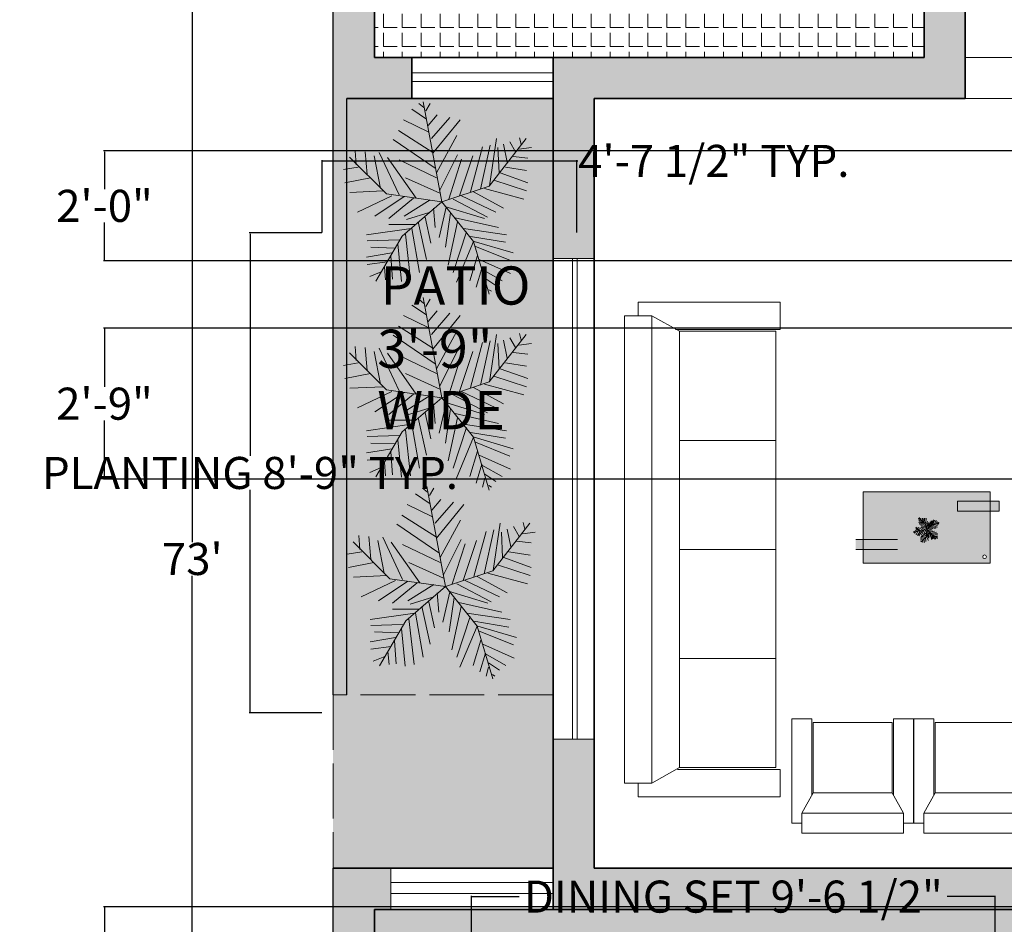
# Model space of a CAD drawing. Units: inches. Extents: x 1884 to 2398, y 474 to 1488.
# Tile 32 of 39: x 1884 to 2099, y 889 to 1087. Entities that reach past the tile are written whole.
import ezdxf

# ---------------------------------------------------------------- set-up
doc = ezdxf.new("R2010")
doc.units = ezdxf.units.IN
doc.header["$MEASUREMENT"] = 0
doc.linetypes.add('ACAD_ISO02W100', pattern=[15, 12, -3])
doc.layers.get('0').update_dxf_attribs({"color": 250})
for name, color, linetype, lineweight in [('A-ANNO-DIMS', 2, 'Continuous', 18), ('A-AREA-IDEN', 7, 'Continuous', 18), ('A-FLOR-OVHD', 8, 'ACAD_ISO02W100', 18), ('A-FLOR-PATT', 254, 'Continuous', 13), ('A-FURN-PATT', 253, 'Continuous', 13), ('A-WALL-PATT', 250, 'Continuous', 13), ('C-PROP', 7, 'Continuous', 30), ('furniture', 8, 'Continuous', 18), ('L-PLNT', 73, 'Continuous', 18), ('walls', 7, 'Continuous', 35), ('windows', 4, 'Continuous', 18)]:
    doc.layers.add(name, color=color, linetype=linetype, lineweight=lineweight)
doc.layers.add('L-PVMT-PATT', color=9, linetype='Continuous', lineweight=13, true_color=0xc7c8ca)
doc.styles.get("Standard").update_dxf_attribs({"font": 'arial.ttf'})
doc.dimstyles.get("Standard").update_dxf_attribs({"dimtxt": 7, "dimasz": 0.18, "dimexe": 0.18, "dimexo": 0.0625, "dimgap": 0.09, "dimtad": 0, "dimtih": 1, "dimtoh": 1, "dimzin": 0, "dimdsep": 46, "dimlunit": 3, "dimtxsty": 'Standard', "dimcen": 0.09, "dimadec": 0, "dimazin": 0, "dimtfac": 1, "dimtofl": 0, "dimtmove": 0, "dimatfit": 3, "dimfxl": 1, "dimtolj": 1, "dimtzin": 0, "dimarcsym": 0})

# ---------------------------------------------------------------- blocks, each defined once
blk = doc.blocks.new('*D2')
at = {"layer": 'A-ANNO-DIMS', "color": 0, "lineweight": -2, "transparency": 16777216}
for p, q in [((1920.51, 1406.88), (1921.96, 1406.88)), ((1921.78, 1406.7), (1921.78, 972.55)), ((1921.78, 531.06), (1921.78, 965.22)), ((1920.51, 530.88), (1921.96, 530.88))]:
    blk.add_line(p, q, dxfattribs=at)
at = {"layer": 'A-ANNO-DIMS', "color": 0, "lineweight": 100, "transparency": 16777216}
for points in [[(1921.75, 1406.7), (1921.81, 1406.7), (1921.78, 1406.88)], [(1921.75, 531.06), (1921.81, 531.06), (1921.78, 530.88)]]:
    blk.add_solid(points, dxfattribs=at)
at = {"layer": 'Defpoints', "color": 0, "lineweight": 100, "transparency": 16777216}
for p in [(1920.45, 1406.88), (1920.45, 530.88), (1921.78, 530.88)]:
    blk.add_point(p, dxfattribs=at)
at = {"layer": 'A-ANNO-DIMS', "color": 0, "transparency": 16777216, "insert": (1921.78, 968.88), "char_height": 7, "attachment_point": 5}
blk.add_mtext("\\A1;73'", dxfattribs=at)
blk = doc.blocks.new('tpoy')
at = {"layer": 'furniture'}
h = blk.add_hatch(color=256, dxfattribs=at)
h.dxf.hatch_style = 1
h.paths.add_polyline_path([(278.09, -251.06), (275.9, -251.06), (275.9, -258.19), (278.09, -258.19)])
h.paths.add_polyline_path([(278.09, -249.1), (275.9, -249.1), (275.9, -251.06), (278.09, -251.06)])
h.paths.add_polyline_path([(286.44, -271.28), (284.25, -271.28), (284.25, -278.76), (286.44, -278.76)])
h.paths.add_polyline_path([(286.44, -278.76), (284.25, -278.76), (284.25, -280.38), (286.44, -280.38)])
for p, q in [((275.9, -249.1), (278.09, -249.1)), ((275.9, -258.19), (275.9, -249.1)), ((278.09, -249.1), (278.09, -258.19)), ((273.86, -251.06), (273.86, -278.76)), ((289.38, -251.06), (273.86, -251.06)), ((289.38, -278.76), (289.38, -251.06)), ((278.09, -258.19), (275.9, -258.19)), ((284.25, -280.38), (284.25, -271.28)), ((286.44, -271.28), (286.44, -280.38)), ((273.86, -278.76), (289.38, -278.76))]:
    blk.add_line(p, q, dxfattribs=at)
blk.add_circle((288.03, -252.28), 0.401, dxfattribs=at)
blk = doc.blocks.new('*U20')
for p, q in [((-7.288, 39.707), (-21.778, 46.673)), ((-8.737, 47.138), (-17.069, 52.711)), ((-10.186, 53.64), (-13.084, 55.962)), ((0, 0), (-10.5, 57)), ((-9.099, 51.782), (-6.563, 55.962)), ((-7.65, 43.423), (-2.578, 49.46)), ((-5.839, 35.992), (4.667, 48.067)), ((-5.114, 27.632), (10.463, 46.673)), ((-47.498, 19.737), (-55.83, 18.344)), ((-40.615, 13.7), (-55.105, 10.913)), ((-31.5, 4.5), (-52.5, 25.5)), ((-33.37, 6.269), (-52.207, 5.34)), ((-48.585, 21.131), (-49.309, 29.026)), ((-28.299, 3.483), (-47.86, -5.805)), ((-43.513, 28.561), (-42.427, 15.558)), ((-38.442, 26.239), (-34.819, 7.663)), ((-21.416, 3.018), (-38.079, -8.128)), ((-35.544, 28.097), (-24.314, 3.947)), ((0, 0), (-31.5, 4.5)), ((-14.533, 2.09), (-30.834, 25.31)), ((-15.982, 2.09), (-30.11, -9.521)), ((-3.665, 19.273), (-27.574, 35.527)), ((-5.114, 28.097), (-24.676, 40.636)), ((-24.314, 23.917), (-2.941, 13.7)), ((0, 0), (-22.5, -19.5)), ((-6.563, 1.161), (-21.416, -8.128)), ((-20.691, 13.7), (-1.129, 4.876)), ((-2.941, 16.486), (8.652, 37.85)), ((-1.129, 6.734), (9.014, 26.704)), ((0, 0), (27, 9)), ((0, 0), (18, -22.5)), ((3.942, 1.625), (11.187, 24.381)), ((6.478, 1.625), (26.04, -8.592)), ((10.101, 3.483), (17.708, 26.239)), ((11.187, 3.483), (30.749, -5.805)), ((16.259, 5.805), (23.142, 31.348)), ((18.07, 5.805), (35.096, -3.483)), ((22.055, 7.198), (27.489, 32.277)), ((24.229, 7.663), (46.688, 1.625)), ((27, 9), (48, 36)), ((27.127, 9.056), (31.112, 35.992)), ((29.662, 12.307), (48.137, 6.269)), ((31.836, 30.883), (32.561, 16.486)), ((33.285, 16.486), (48.862, 10.913)), ((35.096, 32.741), (37.27, 22.524)), ((36.183, 19.737), (48.137, 17.88)), ((38.719, 34.134), (41.979, 28.561)), ((40.53, 25.775), (48.862, 24.846)), ((43.791, 29.954), (51.036, 30.883)), ((44.153, 36.456), (45.239, 32.741)), ((-17.431, -15.094), (-42.789, -18.809)), ((-28.299, -29.026), (-42.789, -31.348)), ((-24.314, -21.596), (-42.427, -22.06)), ((-30.834, -34.135), (-42.427, -35.528)), ((-34.457, -39.708), (-40.978, -42.494)), ((-26.849, -26.24), (-40.253, -25.775)), ((-22.5, -19.5), (-37.5, -45)), ((-32.646, -36.921), (-31.921, -44.352)), ((-15.257, -12.772), (-30.11, -12.772)), ((-29.023, -30.884), (-27.936, -43.887)), ((-25.038, -23.918), (-22.865, -45.281)), ((-20.691, -18.345), (-17.793, -44.352)), ((-6.563, -5.805), (-19.967, -9.985)), ((-17.069, -15.094), (-12.721, -40.172)), ((-13.446, -11.378), (-8.737, -32.741)), ((-9.461, -8.592), (-6.201, -23.453)), ((-4.752, -3.483), (-3.665, -14.629)), ((2.493, -3.019), (-1.491, -20.202)), ((1.769, -2.555), (24.229, -9.521)), ((5.029, -6.27), (2.131, -25.775)), ((9.014, -11.378), (3.58, -35.992)), ((14.085, -16.951), (6.478, -40.172)), ((7.565, -9.056), (32.198, -14.629)), ((18.07, -22.524), (8.289, -45.745)), ((12.274, -15.094), (36.907, -18.809)), ((20.244, -30.419), (15.897, -44.816)), ((16.259, -19.738), (36.183, -22.989)), ((18, -22.5), (27, -52.5)), ((18.433, -22.524), (40.53, -29.026)), ((19.157, -25.311), (38.719, -33.206)), ((22.78, -37.85), (19.519, -48.532)), ((21.331, -32.741), (39.081, -40.636)), ((22.78, -38.314), (34.372, -44.816)), ((24.591, -45.745), (23.142, -50.854)), ((24.591, -43.423), (30.749, -47.603)), ((26.764, -49.925), (28.213, -50.854))]:
    blk.add_line(p, q)
blk = doc.blocks.new('Trees - Imperial')
for p, q in [((0, 0), (-10.5, 57)), ((-8.737, 47.138), (-17.069, 52.711)), ((-10.186, 53.64), (-13.084, 55.962)), ((-9.099, 51.782), (-6.563, 55.962)), ((-7.288, 39.707), (-21.778, 46.673)), ((-7.65, 43.423), (-2.578, 49.46)), ((-5.839, 35.992), (4.667, 48.067)), ((-5.114, 27.632), (10.463, 46.673)), ((-5.114, 28.097), (-24.676, 40.636)), ((-3.665, 19.273), (-27.574, 35.527)), ((-2.941, 16.486), (8.652, 37.85)), ((27, 9), (48, 36)), ((27.127, 9.056), (31.112, 35.992)), ((38.719, 34.134), (41.979, 28.561)), ((44.153, 36.456), (45.239, 32.741)), ((-48.585, 21.131), (-49.309, 29.026)), ((-43.513, 28.561), (-42.427, 15.558)), ((-35.544, 28.097), (-24.314, 3.947)), ((16.259, 5.805), (23.142, 31.348)), ((22.055, 7.198), (27.489, 32.277)), ((31.836, 30.883), (32.561, 16.486)), ((35.096, 32.741), (37.27, 22.524)), ((43.791, 29.954), (51.036, 30.883)), ((-31.5, 4.5), (-52.5, 25.5)), ((-38.442, 26.239), (-34.819, 7.663)), ((-14.533, 2.09), (-30.834, 25.31)), ((-24.314, 23.917), (-2.941, 13.7)), ((-1.129, 6.734), (9.014, 26.704)), ((3.942, 1.625), (11.187, 24.381)), ((10.101, 3.483), (17.708, 26.239)), ((40.53, 25.775), (48.862, 24.846)), ((-47.498, 19.737), (-55.83, 18.344)), ((36.183, 19.737), (48.137, 17.88)), ((-40.615, 13.7), (-55.105, 10.913)), ((-20.691, 13.7), (-1.129, 4.876)), ((29.662, 12.307), (48.137, 6.269)), ((33.285, 16.486), (48.862, 10.913)), ((-33.37, 6.269), (-52.207, 5.34)), ((0, 0), (27, 9)), ((18.07, 5.805), (35.096, -3.483)), ((24.229, 7.663), (46.688, 1.625)), ((-28.299, 3.483), (-47.86, -5.805)), ((-21.416, 3.018), (-38.079, -8.128)), ((0, 0), (-31.5, 4.5)), ((-15.982, 2.09), (-30.11, -9.521)), ((0, 0), (-22.5, -19.5)), ((-6.563, 1.161), (-21.416, -8.128)), ((0, 0), (18, -22.5)), ((6.478, 1.625), (26.04, -8.592)), ((11.187, 3.483), (30.749, -5.805)), ((-4.752, -3.483), (-3.665, -14.629)), ((2.493, -3.019), (-1.491, -20.202)), ((1.769, -2.555), (24.229, -9.521)), ((-6.563, -5.805), (-19.967, -9.985)), ((-9.461, -8.592), (-6.201, -23.453)), ((5.029, -6.27), (2.131, -25.775)), ((7.565, -9.056), (32.198, -14.629)), ((-17.431, -15.094), (-42.789, -18.809)), ((-15.257, -12.772), (-30.11, -12.772)), ((-17.069, -15.094), (-12.721, -40.172)), ((-13.446, -11.378), (-8.737, -32.741)), ((9.014, -11.378), (3.58, -35.992)), ((12.274, -15.094), (36.907, -18.809)), ((-24.314, -21.596), (-42.427, -22.06)), ((-22.5, -19.5), (-37.5, -45)), ((-20.691, -18.345), (-17.793, -44.352)), ((14.085, -16.951), (6.478, -40.172)), ((16.259, -19.738), (36.183, -22.989)), ((-26.849, -26.24), (-40.253, -25.775)), ((-25.038, -23.918), (-22.865, -45.281)), ((18.07, -22.524), (8.289, -45.745)), ((18, -22.5), (27, -52.5)), ((18.433, -22.524), (40.53, -29.026)), ((19.157, -25.311), (38.719, -33.206)), ((-28.299, -29.026), (-42.789, -31.348)), ((-29.023, -30.884), (-27.936, -43.887)), ((20.244, -30.419), (15.897, -44.816)), ((21.331, -32.741), (39.081, -40.636)), ((-30.834, -34.135), (-42.427, -35.528)), ((-32.646, -36.921), (-31.921, -44.352)), ((22.78, -37.85), (19.519, -48.532)), ((22.78, -38.314), (34.372, -44.816)), ((-34.457, -39.708), (-40.978, -42.494)), ((24.591, -43.423), (30.749, -47.603)), ((24.591, -45.745), (23.142, -50.854)), ((26.764, -49.925), (28.213, -50.854))]:
    blk.add_line(p, q)
blk = doc.blocks.new('FABRIC SOFA 4S')
at = {"layer": 'furniture'}
for p, q in [((3, 54), (34, 54)), ((3, 51), (3, 54)), ((34, 48), (34, 54)), ((0, -51), (0, 51)), ((6, 51), (0, 51)), ((6, -51), (6, 51)), ((12, 47.63), (6, 51)), ((11.14, 48), (34, 48)), ((33, 23.81), (12, 23.81)), ((33, 0), (12, 0)), ((33, -23.81), (12, -23.81)), ((6, -51), (12, -47.63)), ((11.54, -48), (34, -48)), ((34, -48), (34, -54)), ((6, -51), (0, -51)), ((3, -54), (3, -51)), ((3, -54), (34, -54))]:
    blk.add_line(p, q, dxfattribs=at)
blk.add_lwpolyline([(12, -47.63), (12, 47.63), (33, 47.63), (33, -47.63)], close=True, dxfattribs=at)
blk = doc.blocks.new('FABRIC SOFA 1S')
at = {"layer": 'furniture'}
for p, q in [((3, 18.12), (34, 18.12)), ((3, 15.12), (3, 18.12)), ((34, 12.12), (34, 18.12)), ((0, -15.12), (0, 15.12)), ((6, 15.12), (0, 15.12)), ((6, -15.12), (6, 15.12)), ((12, 11.75), (6, 15.12)), ((11.33, 12.12), (34, 12.12)), ((6, -15.12), (12, -11.75)), ((11.33, -12.12), (34, -12.12)), ((34, -12.12), (34, -18.12)), ((6, -15.12), (0, -15.12)), ((3, -18.12), (3, -15.12)), ((3, -18.12), (34, -18.12))]:
    blk.add_line(p, q, dxfattribs=at)
blk.add_lwpolyline([(12, -11.75), (12, 11.75), (33, 11.75), (33, -11.75)], close=True, dxfattribs=at)
blk = doc.blocks.new('*D35')
at = {"layer": 'A-ANNO-DIMS', "color": 0, "lineweight": -2, "transparency": 16777216}
for p, q in [((1982.72, 878.09), (1982.72, 895.35)), ((1982.9, 895.17), (1993.17, 895.17)), ((2096.86, 895.17), (2086.6, 895.17)), ((2097.04, 878.09), (2097.04, 895.35))]:
    blk.add_line(p, q, dxfattribs=at)
at = {"layer": 'A-ANNO-DIMS', "color": 0, "lineweight": 100, "transparency": 16777216}
for points in [[(1982.9, 895.2), (1982.9, 895.14), (1982.72, 895.17)], [(2096.86, 895.2), (2096.86, 895.14), (2097.04, 895.17)]]:
    blk.add_solid(points, dxfattribs=at)
at = {"layer": 'Defpoints', "color": 0, "lineweight": 100, "transparency": 16777216}
for p in [(2097.04, 895.17), (1982.72, 878.02), (2097.04, 878.02)]:
    blk.add_point(p, dxfattribs=at)
at = {"layer": 'A-ANNO-DIMS', "color": 0, "transparency": 16777216, "insert": (2039.88, 895.17), "char_height": 7, "attachment_point": 5}
blk.add_mtext('\\A1;DINING SET 9\'-6 1/2"', dxfattribs=at)
blk = doc.blocks.new('*D41')
at = {"layer": 'A-ANNO-DIMS', "color": 0, "lineweight": -2, "transparency": 16777216}
for p, q in [((1950.04, 1040.07), (1934.2, 1040.07)), ((1934.38, 1039.89), (1934.38, 991.37)), ((1934.38, 935.44), (1934.38, 983.96)), ((1950.04, 935.26), (1934.2, 935.26))]:
    blk.add_line(p, q, dxfattribs=at)
at = {"layer": 'A-ANNO-DIMS', "color": 0, "lineweight": 100, "transparency": 16777216}
for points in [[(1934.35, 1039.89), (1934.41, 1039.89), (1934.38, 1040.07)], [(1934.35, 935.44), (1934.41, 935.44), (1934.38, 935.26)]]:
    blk.add_solid(points, dxfattribs=at)
at = {"layer": 'Defpoints', "color": 0, "lineweight": 100, "transparency": 16777216}
for p in [(1934.38, 1040.07), (1950.1, 1040.07), (1950.1, 935.26)]:
    blk.add_point(p, dxfattribs=at)
at = {"layer": 'A-ANNO-DIMS', "color": 0, "transparency": 16777216, "insert": (1934.38, 987.66), "char_height": 7, "attachment_point": 5}
blk.add_mtext('\\A1;PLANTING 8\'-9" TYP.', dxfattribs=at)
blk = doc.blocks.new('*D42')
at = {"layer": 'A-ANNO-DIMS', "color": 0, "lineweight": -2, "transparency": 16777216}
for p, q in [((1950.1, 1040.13), (1950.1, 1055.97)), ((1950.28, 1055.79), (2005.55, 1055.79)), ((2005.73, 1040.13), (2005.73, 1055.97)), ((2005.73, 1055.79), (2005.91, 1055.79))]:
    blk.add_line(p, q, dxfattribs=at)
at = {"layer": 'A-ANNO-DIMS', "color": 0, "lineweight": 100, "transparency": 16777216}
for points in [[(1950.28, 1055.82), (1950.28, 1055.76), (1950.1, 1055.79)], [(2005.55, 1055.82), (2005.55, 1055.76), (2005.73, 1055.79)]]:
    blk.add_solid(points, dxfattribs=at)
at = {"layer": 'Defpoints', "color": 0, "lineweight": 100, "transparency": 16777216}
for p in [(2005.73, 1055.79), (1950.1, 1040.07), (2005.73, 1040.07)]:
    blk.add_point(p, dxfattribs=at)
at = {"layer": 'A-ANNO-DIMS', "color": 0, "transparency": 16777216, "insert": (2035.63, 1055.79), "char_height": 7, "attachment_point": 5}
blk.add_mtext('\\A1;4\'-7 1/2" TYP.', dxfattribs=at)
blk = doc.blocks.new('*D48')
at = {"layer": 'A-ANNO-DIMS', "color": 0, "lineweight": -2, "transparency": 16777216}
for p, q in [((2222.47, 1057.97), (1902.43, 1057.97)), ((1902.61, 1057.79), (1902.61, 1049.64)), ((1902.61, 1034.16), (1902.61, 1042.31)), ((2220.98, 1033.98), (1902.43, 1033.98))]:
    blk.add_line(p, q, dxfattribs=at)
at = {"layer": 'A-ANNO-DIMS', "color": 0, "lineweight": 100, "transparency": 16777216}
for points in [[(1902.58, 1057.79), (1902.64, 1057.79), (1902.61, 1057.97)], [(1902.58, 1034.16), (1902.64, 1034.16), (1902.61, 1033.98)]]:
    blk.add_solid(points, dxfattribs=at)
at = {"layer": 'Defpoints', "color": 0, "lineweight": 100, "transparency": 16777216}
for p in [(1902.61, 1057.97), (2222.53, 1057.97), (2221.05, 1033.98)]:
    blk.add_point(p, dxfattribs=at)
at = {"layer": 'A-ANNO-DIMS', "color": 0, "transparency": 16777216, "insert": (1902.61, 1045.97), "char_height": 7, "attachment_point": 5}
blk.add_mtext('\\A1;2\'-0"', dxfattribs=at)
blk = doc.blocks.new('*D50')
at = {"layer": 'A-ANNO-DIMS', "color": 0, "lineweight": -2, "transparency": 16777216}
for p, q in [((2319.85, 1019.28), (1902.43, 1019.28)), ((1902.61, 1019.1), (1902.61, 1006.44)), ((1902.61, 986.46), (1902.61, 999.11)), ((2319.85, 986.28), (1902.43, 986.28))]:
    blk.add_line(p, q, dxfattribs=at)
at = {"layer": 'A-ANNO-DIMS', "color": 0, "lineweight": 100, "transparency": 16777216}
for points in [[(1902.58, 1019.1), (1902.64, 1019.1), (1902.61, 1019.28)], [(1902.58, 986.46), (1902.64, 986.46), (1902.61, 986.28)]]:
    blk.add_solid(points, dxfattribs=at)
at = {"layer": 'Defpoints', "color": 0, "lineweight": 100, "transparency": 16777216}
for p in [(1902.61, 1019.28), (2319.91, 1019.28), (2319.91, 986.28)]:
    blk.add_point(p, dxfattribs=at)
at = {"layer": 'A-ANNO-DIMS', "color": 0, "transparency": 16777216, "insert": (1902.61, 1002.78), "char_height": 7, "attachment_point": 5}
blk.add_mtext('\\A1;2\'-9"', dxfattribs=at)
blk = doc.blocks.new('*D51')
at = {"layer": 'A-ANNO-DIMS', "color": 0, "lineweight": -2, "transparency": 16777216}
for p, q in [((2202.97, 892.97), (1902.43, 892.97)), ((1902.61, 892.79), (1902.61, 874.82)), ((1902.61, 849.42), (1902.61, 867.39)), ((2202.97, 849.24), (1902.43, 849.24))]:
    blk.add_line(p, q, dxfattribs=at)
at = {"layer": 'A-ANNO-DIMS', "color": 0, "lineweight": 100, "transparency": 16777216}
for points in [[(1902.58, 892.79), (1902.64, 892.79), (1902.61, 892.97)], [(1902.58, 849.42), (1902.64, 849.42), (1902.61, 849.24)]]:
    blk.add_solid(points, dxfattribs=at)
at = {"layer": 'Defpoints', "color": 0, "lineweight": 100, "transparency": 16777216}
for p in [(1902.61, 892.97), (2203.03, 892.97), (2203.03, 849.24)]:
    blk.add_point(p, dxfattribs=at)
at = {"layer": 'A-ANNO-DIMS', "color": 0, "transparency": 16777216, "insert": (1902.61, 871.1), "char_height": 7, "attachment_point": 5}
blk.add_mtext('\\A1;3\'-7 1/2"', dxfattribs=at)

msp = doc.modelspace()

# ---------------------------------------------------------------- hatches: boundary and pattern name
at = {"layer": 'A-FLOR-PATT'}
h = msp.add_hatch(color=256, dxfattribs=at)
h.dxf.hatch_style = 1
h.paths.add_polyline_path([(2117.529, 815.801), (2126.529, 815.801), (2126.529, 880.382), (2117.529, 880.382), (2117.529, 892.385), (1961.529, 892.385), (1961.529, 756.915), (1964.529, 756.915), (1964.529, 759.915), (1995.529, 759.915), (1995.529, 753.915), (1972.862, 753.915), (1967.529, 756.915), (1967.529, 654.915), (1972.862, 657.915), (1995.529, 657.915), (1995.529, 651.915), (1964.529, 651.915), (1964.529, 654.915), (1961.529, 654.915), (1961.529, 640.385), (2117.529, 640.385), (2117.529, 646.578), (2126.529, 646.578), (2126.529, 676.183), (2117.529, 676.183)])
h.paths.add_polyline_path([(2012.246, 808.929), (2012.05, 810.185), (2032.542, 810.185), (2032.346, 808.929)], flags=16)
h.paths.add_polyline_path([(2010.381, 820.864), (1994.658, 820.864), (1994.658, 831.561), (1984.608, 833.132), (1984.608, 853.821), (1994.658, 855.391), (1994.658, 866.089), (2010.381, 866.089), (2011.951, 876.139), (2032.64, 876.139), (2034.211, 866.089), (2045.556, 866.089), (2047.127, 876.139), (2067.816, 876.139), (2069.386, 866.089), (2085.109, 866.089), (2085.109, 855.391), (2095.159, 853.821), (2095.159, 833.132), (2085.109, 831.561), (2085.109, 820.864), (2069.386, 820.864), (2067.816, 810.814), (2047.127, 810.814), (2045.556, 820.864), (2034.211, 820.864), (2032.64, 810.814), (2011.951, 810.814)], flags=16)
h.paths.add_polyline_path([(1982.724, 833.426), (1982.724, 853.526), (1983.98, 853.723), (1983.98, 833.23)], flags=16)
h.paths.add_polyline_path([(1994.529, 753.54), (1994.529, 658.29), (1973.529, 658.29), (1973.529, 753.54)], flags=16)
h.paths.add_polyline_path([(2084.486, 843.527), (2084.592, 843.502), (2084.681, 843.487), (2084.813, 843.477), (2084.913, 843.477), (2084.669, 843.482), (2084.336, 843.565), (2084.116, 843.617), (2083.8, 843.686), (2083.105, 843.827), (2082.836, 843.874), (2083.604, 843.729), (2084.206, 843.597)], flags=0)
h.paths.add_polyline_path([(2047.421, 808.929), (2047.225, 810.185), (2067.718, 810.185), (2067.521, 808.929)], flags=16)
h.paths.add_polyline_path([(2066.01, 849.505), (2066.429, 849.687), (2066.798, 849.882), (2067.129, 850.085), (2067.43, 850.293), (2067.711, 850.502), (2068.176, 850.856), (2068.689, 851.205), (2069.305, 851.531), (2070.015, 851.784), (2070.844, 851.944), (2071.081, 851.956), (2070.629, 851.902), (2070.212, 851.822), (2069.827, 851.717), (2069.471, 851.59), (2069.139, 851.443), (2068.828, 851.279), (2068.534, 851.1), (2068.254, 850.909), (2067.983, 850.709), (2067.502, 850.343), (2066.951, 849.962), (2066.224, 849.579)], flags=0)
h.paths.add_polyline_path([(2059.423, 853.221), (2059.827, 853.278), (2060.171, 853.358), (2060.465, 853.463), (2060.714, 853.589), (2060.926, 853.736), (2061.107, 853.902), (2061.258, 854.086), (2061.377, 854.284), (2061.462, 854.495), (2061.514, 854.715), (2061.53, 854.943), (2061.508, 855.176), (2061.449, 855.411), (2061.352, 855.646), (2061.224, 855.882), (2061.07, 856.117), (2060.9, 856.353), (2060.719, 856.588), (2060.406, 856.993), (2060.103, 857.424), (2059.858, 857.888), (2059.691, 858.467), (2059.836, 859.091), (2060.305, 859.532), (2060.844, 859.798), (2061.513, 859.935), (2062.253, 859.905), (2062.483, 859.849), (2062.078, 859.912), (2061.695, 859.928), (2061.336, 859.899), (2061.005, 859.831), (2060.703, 859.729), (2060.437, 859.597), (2060.208, 859.441), (2060.021, 859.265), (2059.879, 859.075), (2059.785, 858.874), (2059.737, 858.664), (2059.73, 858.447), (2059.761, 858.224), (2059.827, 857.996), (2059.923, 857.765), (2060.047, 857.53), (2060.193, 857.295), (2060.359, 857.06), (2060.537, 856.824), (2060.867, 856.399), (2061.171, 855.978), (2061.422, 855.518), (2061.567, 854.943), (2061.41, 854.272), (2060.947, 853.707), (2060.335, 853.397), (2059.649, 853.236)], flags=0)
h.paths.add_polyline_path([(2050.778, 859.745), (2051.07, 859.87), (2051.295, 860.017), (2051.467, 860.183), (2051.594, 860.365), (2051.679, 860.56), (2051.726, 860.763), (2051.739, 860.971), (2051.722, 861.18), (2051.677, 861.387), (2051.609, 861.587), (2051.521, 861.779), (2051.421, 861.962), (2051.312, 862.138), (2051.203, 862.307), (2050.966, 862.68), (2050.793, 863.193), (2051.021, 863.699), (2051.483, 864.018), (2052.09, 864.138), (2052.773, 864.157), (2053.007, 864.142), (2052.603, 864.152), (2052.258, 864.142), (2051.965, 864.113), (2051.716, 864.064), (2051.504, 863.995), (2051.322, 863.907), (2051.17, 863.802), (2051.048, 863.682), (2050.954, 863.55), (2050.891, 863.408), (2050.856, 863.259), (2050.851, 863.105), (2050.876, 862.948), (2050.929, 862.791), (2051.005, 862.633), (2051.098, 862.472), (2051.203, 862.307), (2051.312, 862.138), (2051.556, 861.742), (2051.751, 861.167), (2051.712, 860.535), (2051.398, 860.085), (2050.949, 859.79)], flags=0)
h.paths.add_polyline_path([(2022.768, 719.264), (2050.461, 719.264), (2050.461, 717.226), (2052.426, 717.226), (2052.426, 715.033), (2050.461, 715.033), (2050.461, 703.738), (2022.768, 703.738)], flags=16)
h.paths.add_polyline_path([(2012.246, 878.023), (2032.346, 878.023), (2032.542, 876.767), (2012.05, 876.767)], flags=16)
h.paths.add_polyline_path([(2035.324, 713.103), (2035.342, 713.294), (2035.192, 713.202)], flags=0)
h.paths.add_polyline_path([(2036.484, 711.63), (2036.583, 711.849), (2036.39, 711.898)], flags=0)
h.paths.add_polyline_path([(2036.074, 712.744), (2035.993, 712.481), (2035.724, 712.516), (2035.794, 712.726)], flags=0)
h.paths.add_polyline_path([(2035.846, 710.909), (2035.753, 710.958), (2035.702, 710.88)], flags=0)
h.paths.add_polyline_path([(2037.818, 712.019), (2037.948, 712.06), (2037.987, 712.161), (2037.815, 712.02)], flags=0)
h.paths.add_polyline_path([(2038.451, 709.517), (2038.464, 709.428), (2038.586, 709.442)], flags=0)
h.paths.add_polyline_path([(2037.805, 709.806), (2037.818, 709.807), (2037.804, 709.823)], flags=0)
h.paths.add_polyline_path([(2036.7, 711.245), (2036.698, 711.236), (2036.813, 711.211)], flags=0)
h.paths.add_polyline_path([(2035.928, 708.897), (2035.668, 708.871), (2035.706, 708.667)], flags=0)
h.paths.add_polyline_path([(2036.414, 710.976), (2035.932, 709.859), (2036.792, 710.484), (2036.5, 710.934)], flags=0)
h.paths.add_polyline_path([(2038.298, 712.115), (2038.499, 712.058), (2038.612, 712.269), (2038.39, 712.332)], flags=0)
h.paths.add_polyline_path([(2047.421, 878.023), (2067.521, 878.023), (2067.718, 876.767), (2047.225, 876.767)], flags=16)
h.paths.add_polyline_path([(2049.647, 705.093, -1), (2048.845, 705.093, -1)], flags=0)
h.paths.add_polyline_path([(2095.787, 853.723), (2097.043, 853.526), (2097.043, 833.426), (2095.787, 833.23)], flags=16)
h.paths.add_polyline_path([(2110.739, 745.339), (2111.75, 745.339, -0.0640419), (2113.267, 742.92), (2113.267, 732.192), (2113.526, 732.192, -0.4142136), (2114.278, 731.439), (2114.278, 716.764, -0.4142136), (2113.526, 716.011), (2113.267, 716.011), (2113.267, 705.284, -0.0640419), (2111.75, 702.864), (2110.739, 702.864), (2110.739, 716.011), (2109.469, 716.011, -0.4142136), (2108.716, 716.764), (2108.716, 731.439, -0.4142136), (2109.469, 732.192), (2110.739, 732.192)], flags=16)
h.paths.add_polyline_path([(1998.045, 668.909), (2002.449, 668.909), (2002.449, 652.273), (2002.724, 652.763), (2002.724, 668.175), (2019.972, 668.175), (2019.972, 652.763), (2020.247, 652.273), (2020.247, 668.909), (2024.651, 668.909), (2029.055, 668.909), (2029.055, 652.273), (2029.33, 652.763), (2029.33, 668.175), (2046.578, 668.175), (2046.578, 652.763), (2046.853, 652.273), (2046.853, 668.909), (2051.257, 668.909), (2051.257, 646.157), (2049.055, 646.157), (2049.055, 643.955), (2026.853, 643.955), (2026.853, 646.157), (2024.651, 646.157), (2022.449, 646.157), (2022.449, 643.955), (2000.247, 643.955), (2000.247, 646.157), (1998.045, 646.157)], flags=16)
h.paths.add_polyline_path([(2342.529, 1247.885), (2265.892, 1247.885), (2230.029, 1247.885), (2209.755, 1247.885), (2168.6, 1247.885), (2168.6, 1104.929), (2158.029, 1104.929), (2158.029, 1079.411), (2168.6, 1079.411), (2168.6, 1062.466), (2342.529, 1062.466), (2342.529, 1093.809)])
h.paths.add_polyline_path([(2215.03, 1153.876), (2215.03, 1164.739), (2187.559, 1164.739), (2187.442, 1152.641), (2173.568, 1152.641), (2173.684, 1164.739), (2173.684, 1218.739), (2173.801, 1230.837), (2187.675, 1230.837), (2187.559, 1218.739), (2215.03, 1218.739), (2215.03, 1225.879), (2245.053, 1225.879), (2245.053, 1153.876)], flags=16)
h.paths.add_polyline_path([(2192.147, 1164.797), (2184.963, 1174.54), (2184.915, 1174.54), (2176.755, 1174.54), (2176.755, 1190.363), (2184.915, 1190.363), (2184.915, 1196.819), (2176.755, 1196.819), (2176.755, 1212.641), (2184.915, 1212.641), (2184.915, 1174.606), (2184.963, 1174.54), (2192.147, 1174.54)], flags=0)
h.paths.add_polyline_path([(2184.971, 1158.364, -1), (2176.039, 1158.364, -1)], flags=0)
h.paths.add_polyline_path([(2335.555, 1161.985), (2335.555, 1175.132), (2334.285, 1175.132, -0.4142136), (2333.533, 1175.885), (2333.533, 1190.56, -0.4142136), (2334.285, 1191.313), (2335.555, 1191.313), (2335.555, 1204.46), (2336.567, 1204.46, -0.0640419), (2338.083, 1202.04), (2338.083, 1191.313), (2338.342, 1191.313, -0.4142136), (2339.095, 1190.56), (2339.095, 1175.885, -0.4142136), (2338.342, 1175.132), (2338.083, 1175.132), (2338.083, 1164.405, -0.0640419), (2336.567, 1161.985)], flags=16)
h.paths.add_polyline_path([(2176.155, 1224.462, -1), (2185.087, 1224.462, -1)], flags=0)
h.paths.add_polyline_path([(2158.029, 1276.197), (2158.029, 1322.885), (2148.233, 1322.885), (2092.029, 1322.885), (1961.529, 1322.885), (1961.529, 1166.885), (2116.005, 1166.885), (2116.005, 1157.885), (2152.638, 1157.885), (2152.638, 1166.885), (2158.029, 1166.885)])
h.paths.add_polyline_path([(2006.352, 1204.245), (2006.352, 1215.108), (1978.881, 1215.108), (1978.764, 1203.01), (1964.89, 1203.01), (1965.006, 1215.108), (1965.006, 1269.108), (1965.123, 1281.207), (1978.997, 1281.207), (1978.881, 1269.108), (2006.352, 1269.108), (2006.352, 1276.248), (2036.375, 1276.248), (2036.375, 1204.245)], flags=16)
h.paths.add_polyline_path([(1983.469, 1215.166), (1976.285, 1224.909), (1976.237, 1224.909), (1968.077, 1224.909), (1968.077, 1240.732), (1976.237, 1240.732), (1976.237, 1247.188), (1968.077, 1247.188), (1968.077, 1263.011), (1976.237, 1263.011), (1976.237, 1224.975), (1976.285, 1224.909), (1983.469, 1224.909)], flags=0)
h.paths.add_polyline_path([(1976.293, 1208.733, -1), (1967.361, 1208.733, -1)], flags=0)
h.paths.add_polyline_path([(1967.477, 1274.832, -1), (1976.41, 1274.832, -1)], flags=0)
h.paths.add_polyline_path([(2152.587, 1223.485), (2152.587, 1236.632), (2151.317, 1236.632, -0.4142136), (2150.564, 1237.385), (2150.564, 1252.06, -0.4142136), (2151.317, 1252.813), (2152.587, 1252.813), (2152.587, 1265.959), (2153.598, 1265.959, -0.0640419), (2155.115, 1263.54), (2155.115, 1252.813), (2155.374, 1252.813, -0.4142136), (2156.126, 1252.06), (2156.126, 1237.385, -0.4142136), (2155.374, 1236.632), (2155.115, 1236.632), (2155.115, 1225.904, -0.0640419), (2153.598, 1223.485)], flags=16)
h.paths.add_polyline_path([(2250.676, 1161.101), (2322.077, 1161.101), (2322.077, 1173.886), (2250.676, 1173.886)], flags=24)
h.paths.add_polyline_path([(2255.61, 1173.712), (2320.136, 1173.712), (2320.136, 1186.659), (2255.61, 1186.659)], flags=24)
h.paths.add_polyline_path([(2053.687, 1230.837), (2125.089, 1230.837), (2125.089, 1243.622), (2053.687, 1243.622)], flags=24)
h.paths.add_polyline_path([(2058.622, 1243.448), (2123.147, 1243.448), (2123.147, 1256.395), (2058.622, 1256.395)], flags=24)
h = msp.add_hatch(dxfattribs=at)
h.set_pattern_fill('ANGLE', color=256, scale=15)
h.set_pattern_definition([(0, (0, 0), (0, 4.125), [3, -1.125]), (90, (0, 0), (-4.125, 3e-16), [3, -1.125])])
h.paths.add_polyline_path([(2081.529, 1122.635), (2090.529, 1122.635), (2090.529, 1152.292), (2081.529, 1152.292), (2081.529, 1162.385), (1961.529, 1162.385), (1961.529, 1078.385), (2081.529, 1078.385)])
at = {"layer": 'A-FURN-PATT'}
h = msp.add_hatch(color=256, dxfattribs=at)
h.dxf.hatch_style = 1
h.paths.add_polyline_path([(2095.939, 979.291), (2088.814, 979.291), (2088.814, 981.485), (2095.939, 981.485), (2095.939, 983.522), (2068.247, 983.522), (2068.247, 973.132), (2075.717, 973.132), (2075.717, 970.939), (2068.247, 970.939), (2068.247, 967.997), (2095.939, 967.997)])
h.paths.add_polyline_path([(2084.086, 976.529), (2084.091, 976.527), (2084.093, 976.531)], flags=16)
h.paths.add_polyline_path([(2082.157, 975.336), (2080.724, 975.046), (2080.734, 975.063), (2080.749, 975.051), (2082.157, 975.336), (2081.674, 976.707), (2081.664, 976.715), (2081.672, 976.714), (2082.157, 975.336), (2082.292, 975.447), (2082.298, 975.468), (2082.313, 975.465), (2082.157, 975.336), (2082.93, 974.475), (2082.941, 974.477), (2082.943, 974.46)], flags=16)
h.paths.add_polyline_path([(2095.126, 969.351, -1), (2094.324, 969.351, -1)], flags=16)
at = {"layer": 'A-WALL-PATT'}
h = msp.add_hatch(color=256, dxfattribs=at)
h.dxf.hatch_style = 1
h.paths.add_polyline_path([(2092.029, 1406.885), (1952.529, 1406.885), (1952.529, 939.249), (1955.529, 939.249), (1955.529, 1069.385), (1969.695, 1069.385), (1969.695, 1078.385), (1961.529, 1078.385), (1961.529, 1397.885), (2087.529, 1397.885), (2087.529, 1322.885), (2092.029, 1322.885), (2092.029, 1328.623)])
h.paths.add_polyline_path([(2087.529, 1345.919), (2014.612, 1345.919), (2014.612, 1327.385), (2007.132, 1327.385), (2007.132, 1322.885), (2019.112, 1322.885), (2019.112, 1327.385), (2019.112, 1341.419), (2087.529, 1341.419)], flags=17)
h.paths.add_polyline_path([(1965.066, 1327.561), (1961.529, 1327.561), (1961.529, 1322.885), (1965.066, 1322.885)], flags=17)
h.paths.add_polyline_path([(2351.529, 1343.885), (2265.892, 1343.885), (2164.726, 1343.885), (2158.029, 1343.885), (2158.029, 1334.885), (2158.029, 1328.623), (2148.233, 1328.623), (2148.233, 1322.885), (2158.029, 1322.885), (2158.029, 1276.197), (2158.029, 1166.885), (2152.638, 1166.885), (2152.638, 1157.885), (2158.029, 1157.885), (2158.029, 1104.929), (2168.6, 1104.929), (2168.6, 1247.885), (2209.755, 1247.885), (2209.755, 1252.385), (2167.029, 1252.385), (2167.029, 1334.885), (2265.892, 1334.885), (2342.529, 1334.885), (2342.529, 1310.041), (2351.529, 1310.041)])
h.paths.add_polyline_path([(2234.529, 1334.885), (2230.029, 1334.885), (2230.029, 1275.554), (2234.529, 1275.554)], flags=17)
h.paths.add_polyline_path([(2342.529, 1252.385), (2265.892, 1252.385), (2234.529, 1252.385), (2234.529, 1256.117), (2230.029, 1256.117), (2230.029, 1247.885), (2265.892, 1247.885), (2342.529, 1247.885)], flags=17)
h.paths.add_polyline_path([(2351.529, 1276.197), (2351.529, 1293.635), (2342.529, 1293.635), (2342.529, 1252.385), (2342.529, 1225.302), (2346.311, 1225.302), (2351.529, 1225.302)], flags=17)
h.paths.add_polyline_path([(2351.529, 1126.264), (2342.529, 1126.264), (2342.529, 1093.809), (2342.529, 1062.466), (2168.6, 1062.466), (2168.6, 1079.411), (2158.029, 1079.411), (2158.029, 1056.803), (2158.029, 1053.466), (2213.529, 1053.466), (2213.529, 934.675), (2222.529, 934.675), (2222.529, 1057.966), (2342.529, 1057.966), (2342.529, 1027.206), (2345.987, 1027.206), (2351.529, 1027.206)])
h.paths.add_polyline_path([(2116.005, 1166.885), (1961.529, 1166.885), (1961.529, 1162.385), (2081.529, 1162.385), (2081.529, 1152.292), (2090.529, 1152.292), (2090.529, 1157.885), (2116.005, 1157.885)])
h.paths.add_polyline_path([(2090.529, 1122.635), (2081.529, 1122.635), (2081.529, 1078.385), (2000.529, 1078.385), (2000.529, 1069.385), (2000.529, 1034.463), (2003.893, 1034.463), (2009.529, 1034.463), (2009.529, 1069.385), (2090.529, 1069.385)], flags=17)
h.paths.add_polyline_path([(2351.529, 974.676), (2342.529, 974.676), (2342.529, 951.86), (2351.529, 951.86)], flags=17)
h = msp.add_hatch(color=256, dxfattribs=at)
h.dxf.hatch_style = 1
h.paths.add_polyline_path([(2351.529, 837.963), (2342.529, 837.963), (2342.529, 813.478), (2351.529, 813.478)])
h.paths.add_polyline_path([(2351.529, 782.175), (2342.529, 782.175), (2342.529, 778.966), (2238.447, 778.966), (2238.447, 769.966), (2351.529, 769.966)])
h.paths.add_polyline_path([(2351.529, 914.773), (2342.529, 914.773), (2342.529, 901.966), (2222.529, 901.966), (2222.529, 908.236), (2213.529, 908.236), (2213.529, 901.966), (2198.529, 901.966), (2198.529, 892.966), (2198.529, 815.857), (2203.029, 815.857), (2203.029, 892.966), (2342.529, 892.966), (2342.529, 869.555), (2346.047, 869.555), (2351.529, 869.555), (2351.529, 880.385)])
h.paths.add_polyline_path([(2208.948, 778.966), (2203.029, 778.966), (2203.029, 782.647), (2198.529, 782.647), (2198.529, 779.109), (2193.526, 779.109), (2193.526, 769.966), (2198.529, 769.966), (2208.948, 769.966)])
h.paths.add_polyline_path([(2126.529, 815.801), (2117.529, 815.801), (2117.529, 676.183), (2126.529, 676.183), (2126.529, 769.966), (2132.515, 769.966), (2132.515, 778.664), (2126.529, 778.664)])
h.paths.add_polyline_path([(2135.996, 901.385), (2009.529, 901.385), (2009.529, 929.544), (2000.529, 929.544), (2000.529, 892.385), (2117.529, 892.385), (2117.529, 880.382), (2126.529, 880.382), (2126.529, 892.385), (2135.996, 892.385)])
h.paths.add_polyline_path([(2198.529, 901.385), (2185.2, 901.385), (2185.2, 892.385), (2198.529, 892.385), (2198.529, 892.966)])
h.paths.add_polyline_path([(1961.529, 892.385), (1965.143, 892.385), (1965.143, 901.385), (1952.529, 901.385), (1952.529, 604.13), (1961.529, 604.13), (1961.529, 631.385), (1988.002, 631.385), (1988.002, 640.385), (1961.529, 640.385)])
h.paths.add_polyline_path([(1955.529, 604.13), (1952.529, 604.13), (1952.529, 530.885), (2126.529, 530.885), (2126.529, 533.885), (1955.529, 533.885)])
h.paths.add_polyline_path([(2396.529, 604.13), (2393.529, 604.13), (2393.529, 533.885), (2126.529, 533.885), (2126.529, 530.885), (2396.529, 530.885)])
h.paths.add_polyline_path([(2396.529, 779.322), (2387.529, 779.322), (2387.529, 604.13), (2396.529, 604.13)])
at = {"layer": 'L-PVMT-PATT'}
h = msp.add_hatch(color=256, dxfattribs=at)
h.dxf.hatch_style = 1
h.paths.add_polyline_path([(2000.529, 1034.463), (2000.529, 1069.385), (1969.695, 1069.385), (1955.529, 1069.385), (1955.529, 939.249), (2000.529, 939.249)])
h = msp.add_hatch(color=256, dxfattribs=at)
h.dxf.hatch_style = 1
h.paths.add_polyline_path([(2000.529, 939.249), (1952.529, 939.249), (1952.529, 901.385), (2000.529, 901.385)])

# ---------------------------------------------------------------- linework, layer by layer
at = {"layer": 'A-FLOR-OVHD'}
for p, q in [((2090.529, 1078.385), (2158.029, 1078.385)), ((2090.529, 1069.385), (2158.029, 1069.385)), ((2000.529, 939.249), (1952.529, 939.249)), ((1952.529, 939.249), (1952.529, 901.385))]:
    msp.add_line(p, q, dxfattribs=at)
at = {"layer": 'C-PROP'}
for p, q in [((1952.529, 939.249), (1952.529, 1406.885)), ((1955.529, 939.249), (1955.529, 1069.385)), ((1952.529, 530.885), (1952.529, 901.385))]:
    msp.add_line(p, q, dxfattribs=at)
at = {"layer": 'walls'}
for p, q in [((1961.529, 1078.385), (1961.529, 1397.885)), ((2090.529, 1069.385), (2090.529, 1157.885)), ((2081.529, 1078.385), (2081.529, 1122.635)), ((1961.529, 1078.385), (2081.529, 1078.385)), ((1969.695, 1078.385), (1969.695, 1069.385)), ((2000.529, 892.385), (2000.529, 1078.385)), ((1955.529, 1069.385), (2000.529, 1069.385)), ((2009.529, 901.385), (2009.529, 1069.385)), ((2009.529, 1069.385), (2090.529, 1069.385)), ((1952.529, 901.385), (2000.529, 901.385)), ((2009.529, 901.385), (2135.996, 901.385)), ((1961.529, 892.385), (2117.529, 892.385)), ((1961.529, 640.385), (1961.529, 892.385))]:
    msp.add_line(p, q, dxfattribs=at)
at = {"layer": 'windows'}
for p, q in [((1969.695, 1078.385), (1969.695, 1069.385)), ((2000.529, 1078.385), (1969.695, 1078.385)), ((1969.695, 1078.385), (1969.695, 1074.978)), ((2000.529, 1069.385), (2000.529, 1078.385)), ((1969.695, 1074.978), (2000.529, 1074.978)), ((2000.529, 1074.978), (2000.529, 1073.151)), ((2000.529, 1073.151), (1969.695, 1073.151)), ((1969.695, 1069.385), (2000.529, 1069.385)), ((2000.529, 1034.463), (2009.529, 1034.463)), ((2000.529, 929.544), (2000.529, 1034.463)), ((2000.529, 1034.463), (2003.893, 1034.463)), ((2004.776, 929.544), (2004.776, 1034.463)), ((2004.776, 1034.463), (2005.179, 1034.463)), ((2005.824, 929.544), (2005.824, 1034.463)), ((2009.529, 1034.463), (2009.529, 929.544)), ((2009.529, 929.544), (2000.529, 929.544)), ((2003.893, 929.544), (2006.683, 929.544)), ((1965.143, 901.385), (1965.143, 892.385)), ((2000.529, 901.385), (1965.143, 901.385)), ((1965.143, 901.385), (1965.143, 898.223)), ((2000.529, 892.385), (2000.529, 901.385)), ((1965.143, 898.223), (2000.529, 898.223)), ((2000.529, 898.223), (2000.529, 895.883)), ((2000.529, 895.883), (1965.143, 895.883)), ((1965.143, 892.385), (2000.529, 892.385))]:
    msp.add_line(p, q, dxfattribs=at)

# ---------------------------------------------------------------- block references
at = {"layer": 'furniture'}
msp.add_blockref('FABRIC SOFA 4S', (2016.134, 970.951), dxfattribs=at)
at = {"layer": 'furniture', "rotation": 270}
msp.add_blockref('tpoy', (2347.002, 1257.38), dxfattribs=at)
at = {"layer": 'furniture', "xscale": -0.7339463821036302, "yscale": 0.7339463821036302, "zscale": 0.7339463821036302}
for p, rotation in [((2065.953, 908.991), 270), ((2092.558, 908.991), 269.9999999999993)]:
    msp.add_blockref('FABRIC SOFA 1S', p, dxfattribs=dict(at, rotation=rotation))
at = {"layer": 'L-PLNT', "xscale": 0.3838579184500575, "yscale": 0.3838579184500575, "zscale": 0.3838579184500575}
for p in [(1976.238, 1046.833), (1976.238, 1004.089), (1977.027, 962.852)]:
    msp.add_blockref('Trees - Imperial', p, dxfattribs=at)
at = {"layer": 'L-PLNT', "xscale": 0.0510892351028333, "yscale": 0.0510892351028333, "zscale": 0.0510892351028333, "rotation": 90.98387132377816}
msp.add_blockref('*U20', (2082.157, 975.336), dxfattribs=at)

# ---------------------------------------------------------------- texts
at = {"layer": 'A-AREA-IDEN'}
for s, p in [('PATIO', (1962.89, 1024.403)), ('3\'-9"', (1962.177, 1010.596)), ('WIDE', (1962.177, 997.216))]:
    msp.add_text(s, height=8.3413, dxfattribs=at).set_placement(p)

# ---------------------------------------------------------------- dimensions: what is measured, and where the dimension line sits
at = {"layer": 'A-ANNO-DIMS'}
for base, p1, p2, override, picture, middle in [((1921.782, 530.885), (1920.445, 1406.885), (1920.445, 530.885), {"dimclrd": 0, "dimclre": 0, "dimclrt": 0}, '*D2', (1921.782, 968.885)), ((1902.612, 1057.966), (2221.046, 1033.976), (2222.529, 1057.966), {"dimdec": 1, "dimlfac": 1, "dimrnd": 0, "dimzin": 1, "dimdsep": 46, "dimlunit": 4, "dimfrac": 2}, '*D48', (1902.612, 1045.971)), ((1902.612, 1019.278), (2319.909, 986.278), (2319.909, 1019.278), {"dimdec": 1, "dimlfac": 1, "dimrnd": 0, "dimzin": 1, "dimdsep": 46, "dimlunit": 4, "dimfrac": 2}, '*D50', (1902.612, 1002.778)), ((1902.612, 892.966), (2203.029, 849.241), (2203.029, 892.966), {"dimdec": 1, "dimlfac": 1, "dimrnd": 0, "dimzin": 1, "dimdsep": 46, "dimlunit": 4, "dimfrac": 2}, '*D51', (1902.612, 871.103))]:
    dim = msp.add_linear_dim(base=base, p1=p1, p2=p2, angle=90, dimstyle='Standard', override=override, dxfattribs=at)
    dim.commit()
    dim.dimension.update_dxf_attribs({"geometry": picture, "text_midpoint": middle})
for base, p1, p2, text, picture, middle in [((2005.726, 1055.794), (1950.101, 1040.072), (2005.726, 1040.072), '<> TYP.', '*D42', (2035.627, 1055.794)), ((2097.043, 895.171), (1982.724, 878.023), (2097.043, 878.023), 'DINING SET <>', '*D35', (2039.884, 895.171))]:
    dim = msp.add_linear_dim(base=base, p1=p1, p2=p2, text=text, dimstyle='Standard', override={"dimdec": 1, "dimlfac": 1, "dimrnd": 0, "dimzin": 1, "dimdsep": 46, "dimlunit": 4, "dimfrac": 2}, dxfattribs=at)
    dim.commit()
    dim.dimension.update_dxf_attribs({"geometry": picture, "text_midpoint": middle})
dim = msp.add_linear_dim(base=(1934.379, 1040.072), p1=(1950.101, 935.258), p2=(1950.101, 1040.072), angle=90, text='PLANTING <> TYP.', dimstyle='Standard', override={"dimdec": 1, "dimlfac": 1, "dimrnd": 0, "dimzin": 1, "dimdsep": 46, "dimlunit": 4, "dimfrac": 2}, dxfattribs=at)
dim.commit()
dim.dimension.update_dxf_attribs({"geometry": '*D41', "text_midpoint": (1934.379, 987.665)})

doc.saveas('drawing.dxf')
